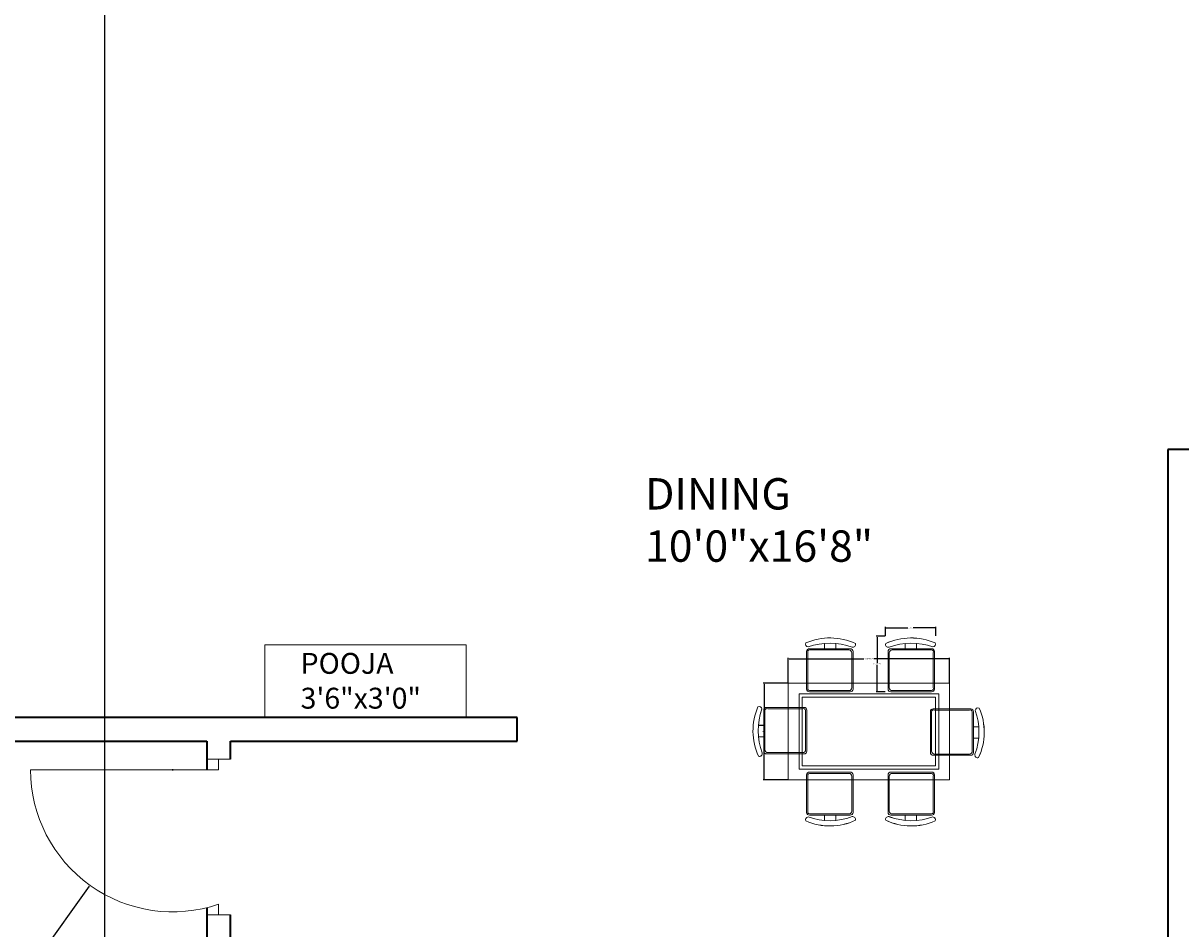
# Model space of a CAD drawing. Units: inches. Extents: x 1902 to 2626, y 1199 to 2408.
# Tile 3 of 9: x 2113 to 2334, y 1470 to 1644. Entities that reach past the tile are written whole.
import ezdxf

# ---------------------------------------------------------------- set-up
doc = ezdxf.new("R2010")
doc.units = ezdxf.units.IN
for name, color, linetype, lineweight in [('A-ANNO-DIMS', 2, 'Continuous', 18), ('A-AREA-IDEN', 7, 'Continuous', 18), ('A-DOOR', 31, 'Continuous', 18), ('A-FLOR-CASE', 8, 'Continuous', 18), ('A-FURN', 8, 'Continuous', 13), ('A-WALL', 7, 'Continuous', 35)]:
    doc.layers.add(name, color=color, linetype=linetype, lineweight=lineweight)
doc.styles.get("Standard").update_dxf_attribs({"font": 'arial.ttf'})
doc.dimstyles.get("Standard").update_dxf_attribs({"dimtxt": 0.18, "dimasz": 0.18, "dimexe": 0.18, "dimexo": 0.0625, "dimgap": 0.09, "dimtad": 0, "dimtih": 1, "dimtoh": 1, "dimdec": 4, "dimzin": 0, "dimdsep": 46, "dimtxsty": 'Standard', "dimcen": 0.09, "dimadec": 0, "dimazin": 0, "dimtfac": 1, "dimtdec": 4, "dimtofl": 0, "dimtmove": 0, "dimatfit": 3, "dimfxl": 1, "dimtolj": 1, "dimtzin": 0, "dimarcsym": 0})

# ---------------------------------------------------------------- blocks, each defined once
blk = doc.blocks.new('TABLE-DINING-RECT')
for points in [[(0, 18.51), (30.84, 18.51), (30.84, 0), (0, 0)], [(2.06, 16.45), (28.79, 16.45), (28.79, 2.06), (2.06, 2.06)], [(2.67, 15.83), (28.17, 15.83), (28.17, 2.67), (2.67, 2.67)]]:
    blk.add_lwpolyline(points, close=True)
blk = doc.blocks.new('CHAIR-DINING')
for points in [[(8.55, 2.06), (0.75, 2.06, -0.414214), (0.2, 2.6), (0.2, 9.77, -0.414214), (0.75, 10.32), (8.55, 10.32, -0.414214), (9.09, 9.77), (9.09, 2.6, -0.414214), (8.55, 2.06)], [(8.91, 1.78, -0.578392), (9.54, 1.08, -0.214524), (0.06, 0.96, -0.552014), (0.5, 1.72, 0.175809), (8.91, 1.78)], [(5.81, 2.06), (5.81, 1.07, 0.064759)]]:
    blk.add_lwpolyline(points, format="xyb")
blk.add_lwpolyline([(0.75, 2.3), (8.3, 2.3, 0.414214), (8.85, 2.85), (8.85, 9.53, 0.414214), (8.3, 10.07), (0.75, 10.07, 0.512069), (0.45, 9.53), (0.45, 2.85, 0.512069)], format="xyb", close=True)
blk.add_lwpolyline([(3.63, 1.05), (3.63, 2.06)])
blk = doc.blocks.new('*D12')
at = {"layer": 'A-ANNO-DIMS', "color": 0, "lineweight": -2, "transparency": 16777216}
for p, q in [((2259.21, 1517.35), (2259.21, 1522.1)), ((2259.39, 1521.92), (2273.67, 1521.92)), ((2289.87, 1521.92), (2275.6, 1521.92)), ((2290.05, 1517.35), (2290.05, 1522.1))]:
    blk.add_line(p, q, dxfattribs=at)
at = {"layer": 'A-ANNO-DIMS', "color": 0, "transparency": 16777216}
for points in [[(2259.39, 1521.95), (2259.39, 1521.89), (2259.21, 1521.92)], [(2289.87, 1521.95), (2289.87, 1521.89), (2290.05, 1521.92)]]:
    blk.add_solid(points, dxfattribs=at)
at = {"layer": 'Defpoints', "color": 0, "transparency": 16777216}
for p in [(2290.05, 1521.92), (2259.21, 1517.29), (2290.05, 1517.29)]:
    blk.add_point(p, dxfattribs=at)
at = {"layer": 'A-ANNO-DIMS', "color": 0, "transparency": 16777216, "insert": (2274.63, 1521.92), "char_height": 0.18, "attachment_point": 5}
blk.add_mtext('\\A1;TABLE 31 TYP.', dxfattribs=at)
blk = doc.blocks.new('*D13')
at = {"layer": 'A-ANNO-DIMS', "color": 0, "lineweight": -2, "transparency": 16777216}
for p, q in [((2259.15, 1517.29), (2254.4, 1517.29)), ((2254.58, 1517.11), (2254.58, 1508.22)), ((2254.58, 1498.96), (2254.58, 1507.85)), ((2259.15, 1498.78), (2254.4, 1498.78))]:
    blk.add_line(p, q, dxfattribs=at)
at = {"layer": 'A-ANNO-DIMS', "color": 0, "transparency": 16777216}
for points in [[(2254.55, 1517.11), (2254.61, 1517.11), (2254.58, 1517.29)], [(2254.55, 1498.96), (2254.61, 1498.96), (2254.58, 1498.78)]]:
    blk.add_solid(points, dxfattribs=at)
at = {"layer": 'Defpoints', "color": 0, "transparency": 16777216}
for p in [(2254.58, 1517.29), (2259.21, 1517.29), (2259.21, 1498.78)]:
    blk.add_point(p, dxfattribs=at)
at = {"layer": 'A-ANNO-DIMS', "color": 0, "transparency": 16777216, "insert": (2254.58, 1508.04), "char_height": 0.18, "attachment_point": 5}
blk.add_mtext('\\A1;19 TYP.', dxfattribs=at)
blk = doc.blocks.new('*D14')
at = {"layer": 'A-ANNO-DIMS', "color": 0, "lineweight": -2, "transparency": 16777216}
for p, q in [((2277.74, 1526.29), (2276.02, 1526.29)), ((2276.2, 1526.11), (2276.2, 1521.13)), ((2276.2, 1515.79), (2276.2, 1520.77)), ((2277.74, 1515.61), (2276.02, 1515.61))]:
    blk.add_line(p, q, dxfattribs=at)
at = {"layer": 'A-ANNO-DIMS', "color": 0, "transparency": 16777216}
for points in [[(2276.17, 1526.11), (2276.23, 1526.11), (2276.2, 1526.29)], [(2276.17, 1515.79), (2276.23, 1515.79), (2276.2, 1515.61)]]:
    blk.add_solid(points, dxfattribs=at)
at = {"layer": 'Defpoints', "color": 0, "transparency": 16777216}
for p in [(2277.8, 1526.29), (2276.2, 1515.61), (2277.8, 1515.61)]:
    blk.add_point(p, dxfattribs=at)
at = {"layer": 'A-ANNO-DIMS', "color": 0, "transparency": 16777216, "insert": (2276.2, 1520.95), "char_height": 0.18, "attachment_point": 5}
blk.add_mtext('\\A1;CHAIR 11 TYP.', dxfattribs=at)
blk = doc.blocks.new('*D15')
at = {"layer": 'A-ANNO-DIMS', "color": 0, "lineweight": -2, "transparency": 16777216}
for p, q in [((2277.8, 1526.35), (2277.8, 1528.07)), ((2277.98, 1527.89), (2282.1, 1527.89)), ((2287.25, 1527.89), (2283.14, 1527.89)), ((2287.43, 1526.35), (2287.43, 1528.07))]:
    blk.add_line(p, q, dxfattribs=at)
at = {"layer": 'A-ANNO-DIMS', "color": 0, "transparency": 16777216}
for points in [[(2277.98, 1527.92), (2277.98, 1527.86), (2277.8, 1527.89)], [(2287.25, 1527.92), (2287.25, 1527.86), (2287.43, 1527.89)]]:
    blk.add_solid(points, dxfattribs=at)
at = {"layer": 'Defpoints', "color": 0, "transparency": 16777216}
for p in [(2277.8, 1527.89), (2277.8, 1526.29), (2287.43, 1526.29)]:
    blk.add_point(p, dxfattribs=at)
at = {"layer": 'A-ANNO-DIMS', "color": 0, "transparency": 16777216, "insert": (2282.62, 1527.89), "char_height": 0.18, "attachment_point": 5}
blk.add_mtext('\\A1;10 TYP.', dxfattribs=at)
blk = doc.blocks.new('*D29')
at = {"layer": 'A-ANNO-DIMS', "color": 0, "lineweight": -2, "transparency": 16777216}
for p, q in [((2191.29, 2322.47), (1943.87, 2322.47)), ((1944.05, 2322.29), (1944.05, 1836.38)), ((1944.05, 1350.11), (1944.05, 1836.02)), ((2202.79, 1349.93), (1943.87, 1349.93))]:
    blk.add_line(p, q, dxfattribs=at)
at = {"layer": 'A-ANNO-DIMS', "color": 0, "transparency": 16777216}
for points in [[(1944.02, 2322.29), (1944.08, 2322.29), (1944.05, 2322.47)], [(1944.02, 1350.11), (1944.08, 1350.11), (1944.05, 1349.93)]]:
    blk.add_solid(points, dxfattribs=at)
at = {"layer": 'Defpoints', "color": 0, "transparency": 16777216}
for p in [(1944.05, 2322.47), (2191.35, 2322.47), (2202.85, 1349.93)]:
    blk.add_point(p, dxfattribs=at)
at = {"layer": 'A-ANNO-DIMS', "color": 0, "transparency": 16777216, "insert": (1944.05, 1836.2), "char_height": 0.18, "attachment_point": 5}
blk.add_mtext('\\A1;972.5', dxfattribs=at)
blk = doc.blocks.new('*D38')
at = {"layer": 'A-ANNO-DIMS', "color": 0, "lineweight": -2, "transparency": 16777216}
for p, q in [((2008.35, 1874.05), (2008.35, 1198.67)), ((2128.35, 1874.05), (2128.35, 1198.67)), ((2008.53, 1198.85), (2068.07, 1198.85)), ((2128.17, 1198.85), (2068.63, 1198.85))]:
    blk.add_line(p, q, dxfattribs=at)
at = {"layer": 'A-ANNO-DIMS', "color": 0, "transparency": 16777216}
for points in [[(2008.53, 1198.88), (2008.53, 1198.82), (2008.35, 1198.85)], [(2128.17, 1198.88), (2128.17, 1198.82), (2128.35, 1198.85)]]:
    blk.add_solid(points, dxfattribs=at)
at = {"layer": 'Defpoints', "color": 0, "transparency": 16777216}
for p in [(2008.35, 1874.11), (2128.35, 1874.11), (2128.35, 1198.85)]:
    blk.add_point(p, dxfattribs=at)
at = {"layer": 'A-ANNO-DIMS', "color": 0, "transparency": 16777216, "insert": (2068.35, 1198.85), "char_height": 0.18, "attachment_point": 5}
blk.add_mtext('\\A1;120', dxfattribs=at)
blk = doc.blocks.new('*D51')
at = {"layer": 'A-ANNO-DIMS', "color": 0, "lineweight": -2, "transparency": 16777216}
for p, q in [((2141.3, 1500.7), (2141.48, 1500.7)), ((2141.39, 1500.61), (2141.39, 1500.79)), ((2116.07, 1465.29), (2125.46, 1478.42)), ((2115.89, 1465.29), (2116.07, 1465.29))]:
    blk.add_line(p, q, dxfattribs=at)
at = {"layer": 'A-ANNO-DIMS', "color": 0, "transparency": 16777216}
blk.add_solid([(2125.44, 1478.44), (2125.49, 1478.4), (2125.57, 1478.57)], dxfattribs=at)
at = {"layer": 'Defpoints', "color": 0, "transparency": 16777216}
for p in [(2141.39, 1500.7), (2125.57, 1478.57)]:
    blk.add_point(p, dxfattribs=at)
at = {"layer": 'A-ANNO-DIMS', "color": 0, "transparency": 16777216, "insert": (2115.34, 1465.29), "char_height": 0.18, "attachment_point": 5}
blk.add_mtext('\\A1;R27.204', dxfattribs=at)

msp = doc.modelspace()

# ---------------------------------------------------------------- linework, layer by layer
at = {"layer": 'A-DOOR'}
for p, q in [((2152.4363, 1502.6974), (2147.9363, 1502.6974)), ((2147.9363, 1502.6974), (2150.1863, 1502.6974)), ((2150.1863, 1502.6974), (2150.1863, 1502.6974)), ((2150.1863, 1502.6974), (2150.1863, 1500.6974)), ((2150.1863, 1500.6974), (2114.1863, 1500.6974)), ((2150.1863, 1472.9548), (2150.1863, 1474.9548)), ((2147.9363, 1472.9548), (2152.4363, 1472.9548)), ((2152.4363, 1472.9548), (2150.1863, 1472.9548))]:
    msp.add_line(p, q, dxfattribs=at)
msp.add_arc((2141.3902, 1500.6974), 27.2039, 180, 288.865006, dxfattribs=at)
at = {"layer": 'A-FLOR-CASE'}
msp.add_lwpolyline([(2159.0496, 1524.6144), (2197.5917, 1524.6144), (2197.5917, 1510.7028), (2159.0496, 1510.7028)], close=True, dxfattribs=at)
at = {"layer": 'A-FURN'}
for points in [[(2263.0262, 1524.2123, -0.17580919), (2271.427, 1524.1486, 0.57839206), (2272.0634, 1524.8484, 0.21452438), (2262.5807, 1524.9757, 0.55201397), (2263.0262, 1524.2123, -0.06507904)], [(2263.0262, 1524.2123, -0.17580919), (2271.427, 1524.1486, 0.57839206), (2272.0634, 1524.8484, 0.21452438), (2262.5807, 1524.9757, 0.55201397), (2263.0262, 1524.2123, -0.06507904)], [(2263.0262, 1524.2119, -0.17580919), (2271.427, 1524.1483, 0.57839206), (2272.0635, 1524.8481, 0.21452438), (2262.5807, 1524.9754, 0.55201397), (2263.0262, 1524.2119, -0.06507904)], [(2263.0262, 1524.2119, -0.17580919), (2271.427, 1524.1483, 0.57839206), (2272.0635, 1524.8481, 0.21452438), (2262.5807, 1524.9754, 0.55201397), (2263.0262, 1524.2119, -0.06507904)], [(2268.3312, 1523.8751), (2268.3312, 1524.8614, -0.06475861)], [(2268.3312, 1523.8751), (2268.3312, 1524.8614, -0.06475861)], [(2268.3312, 1523.8748), (2268.3312, 1524.8611, -0.06475861)], [(2268.3312, 1523.8748), (2268.3312, 1524.8611, -0.06475861)], [(2278.4995, 1524.1486, -0.57839206), (2277.863, 1524.8484, -0.21452438), (2287.3458, 1524.9757, -0.55201397), (2286.9003, 1524.2123, 0.1758092), (2278.4995, 1524.1486)], [(2278.4995, 1524.1486, -0.57839206), (2277.863, 1524.8484, -0.21452438), (2287.3458, 1524.9757, -0.55201397), (2286.9003, 1524.2123, 0.1758092), (2278.4995, 1524.1486)], [(2278.4995, 1524.1483, -0.57839206), (2277.863, 1524.8481, -0.21452438), (2287.3458, 1524.9754, -0.55201397), (2286.9003, 1524.2119, 0.1758092), (2278.4995, 1524.1483)], [(2281.5953, 1523.8751), (2281.5953, 1524.8614, 0.06475861)], [(2281.5953, 1523.8751), (2281.5953, 1524.8614, 0.06475861)], [(2281.5953, 1523.8748), (2281.5953, 1524.8611, 0.06475861)], [(2271.0706, 1523.8751), (2263.2715, 1523.8751, 0.41421356), (2262.7259, 1523.3295), (2262.7259, 1516.1584, 0.41421356), (2263.2715, 1515.6127), (2271.0706, 1515.6127, 0.41421356), (2271.6162, 1516.1584), (2271.6162, 1523.3295, 0.41421356), (2271.0706, 1523.8751)], [(2271.0706, 1523.8751), (2263.2715, 1523.8751, 0.41421356), (2262.7259, 1523.3295), (2262.7259, 1516.1584, 0.41421356), (2263.2715, 1515.6127), (2271.0706, 1515.6127, 0.41421356), (2271.6162, 1516.1584), (2271.6162, 1523.3295, 0.41421356), (2271.0706, 1523.8751)], [(2271.0706, 1523.8748), (2263.2716, 1523.8748, 0.41421356), (2262.7259, 1523.3291), (2262.7259, 1516.158, 0.41421356), (2263.2716, 1515.6124), (2271.0706, 1515.6124, 0.41421356), (2271.6163, 1516.158), (2271.6163, 1523.3291, 0.41421356), (2271.0706, 1523.8748)], [(2271.0706, 1523.8748), (2263.2716, 1523.8748, 0.41421356), (2262.7259, 1523.3291), (2262.7259, 1516.158, 0.41421356), (2263.2716, 1515.6124), (2271.0706, 1515.6124, 0.41421356), (2271.6163, 1516.158), (2271.6163, 1523.3291, 0.41421356), (2271.0706, 1523.8748)], [(2286.6549, 1523.8751, -0.41421356), (2287.2006, 1523.3295), (2287.2006, 1516.1584, -0.41421356), (2286.6549, 1515.6127), (2278.8559, 1515.6127, -0.41421356), (2278.3102, 1516.1584), (2278.3102, 1523.3295, -0.41421356), (2278.8559, 1523.8751), (2286.6549, 1523.8751)], [(2286.6549, 1523.8751, -0.41421356), (2287.2006, 1523.3295), (2287.2006, 1516.1584, -0.41421356), (2286.6549, 1515.6127), (2278.8559, 1515.6127, -0.41421356), (2278.3102, 1516.1584), (2278.3102, 1523.3295, -0.41421356), (2278.8559, 1523.8751), (2286.6549, 1523.8751)], [(2286.6549, 1523.8748, -0.41421356), (2287.2006, 1523.3291), (2287.2006, 1516.158, -0.41421356), (2286.6549, 1515.6124), (2278.8559, 1515.6124, -0.41421356), (2278.3102, 1516.158), (2278.3102, 1523.3291, -0.41421356), (2278.8559, 1523.8748), (2286.6549, 1523.8748)], [(2254.2373, 1503.9255, -0.57839206), (2253.5375, 1503.289, -0.21452438), (2253.4102, 1512.7718, -0.55201397), (2254.1736, 1512.3263, 0.17580937), (2254.2373, 1503.9255)], [(2254.2373, 1503.9255, -0.57839206), (2253.5375, 1503.289, -0.21452438), (2253.4102, 1512.7718, -0.55201397), (2254.1736, 1512.3263, 0.17580937), (2254.2373, 1503.9255)], [(2254.5108, 1512.0809, -0.41421356), (2255.0564, 1512.6266), (2262.2275, 1512.6266, -0.41421356), (2262.7732, 1512.0809), (2262.7732, 1504.2819, -0.41421356), (2262.2275, 1503.7363), (2255.0564, 1503.7363, -0.41421356), (2254.5108, 1504.2819), (2254.5108, 1512.0809)], [(2254.5108, 1512.0809, -0.41421356), (2255.0564, 1512.6266), (2262.2275, 1512.6266, -0.41421356), (2262.7732, 1512.0809), (2262.7732, 1504.2819, -0.41421356), (2262.2275, 1503.7363), (2255.0564, 1503.7363, -0.41421356), (2254.5108, 1504.2819), (2254.5108, 1512.0809)], [(2294.6724, 1511.8135, 0.41421356), (2294.1267, 1512.3592), (2286.9557, 1512.3592, 0.41421356), (2286.41, 1511.8135), (2286.41, 1504.0145, 0.41421356), (2286.9557, 1503.4688), (2294.1267, 1503.4688, 0.41421356), (2294.6724, 1504.0145), (2294.6724, 1511.8135)], [(2295.0095, 1512.0589, -0.17580919), (2294.9459, 1503.658, 0.57839206), (2295.6457, 1503.0216, 0.21452438), (2295.773, 1512.5044, 0.55201397), (2295.0095, 1512.0589, -0.06507904)], [(2254.5108, 1507.0213), (2253.5245, 1507.0213, 0.06475861)], [(2254.5108, 1507.0213), (2253.5245, 1507.0213, 0.06475861)], [(2294.6724, 1506.7539), (2295.6587, 1506.7539, -0.06475861)], [(2271.0706, 1491.9978), (2263.2715, 1491.9978, -0.41421356), (2262.7259, 1492.5435), (2262.7259, 1499.7145, -0.41421356), (2263.2715, 1500.2602), (2271.0706, 1500.2602, -0.41421356), (2271.6162, 1499.7145), (2271.6162, 1492.5435, -0.41421356), (2271.0706, 1491.9978)], [(2271.0706, 1491.9978), (2263.2715, 1491.9978, -0.41421356), (2262.7259, 1492.5435), (2262.7259, 1499.7145, -0.41421356), (2263.2715, 1500.2602), (2271.0706, 1500.2602, -0.41421356), (2271.6162, 1499.7145), (2271.6162, 1492.5435, -0.41421356), (2271.0706, 1491.9978)], [(2271.0706, 1491.9975), (2263.2716, 1491.9975, -0.41421356), (2262.7259, 1492.5431), (2262.7259, 1499.7142, -0.41421356), (2263.2716, 1500.2599), (2271.0706, 1500.2599, -0.41421356), (2271.6163, 1499.7142), (2271.6163, 1492.5431, -0.41421356), (2271.0706, 1491.9975)], [(2271.0706, 1491.9975), (2263.2716, 1491.9975, -0.41421356), (2262.7259, 1492.5431), (2262.7259, 1499.7142, -0.41421356), (2263.2716, 1500.2599), (2271.0706, 1500.2599, -0.41421356), (2271.6163, 1499.7142), (2271.6163, 1492.5431, -0.41421356), (2271.0706, 1491.9975)], [(2286.6549, 1491.9978, 0.41421356), (2287.2006, 1492.5435), (2287.2006, 1499.7145, 0.41421356), (2286.6549, 1500.2602), (2278.8559, 1500.2602, 0.41421356), (2278.3102, 1499.7145), (2278.3102, 1492.5435, 0.41421356), (2278.8559, 1491.9978), (2286.6549, 1491.9978)], [(2286.6549, 1491.9975, 0.41421356), (2287.2006, 1492.5431), (2287.2006, 1499.7142, 0.41421356), (2286.6549, 1500.2599), (2278.8559, 1500.2599, 0.41421356), (2278.3102, 1499.7142), (2278.3102, 1492.5431, 0.41421356), (2278.8559, 1491.9975), (2286.6549, 1491.9975)], [(2271.427, 1491.7243, -0.57839206), (2272.0634, 1491.0245, -0.21452438), (2262.5807, 1490.8972, -0.55201397), (2263.0262, 1491.6607, 0.17580929), (2271.427, 1491.7243)], [(2271.427, 1491.7243, -0.57839206), (2272.0634, 1491.0245, -0.21452438), (2262.5807, 1490.8972, -0.55201397), (2263.0262, 1491.6607, 0.17580929), (2271.427, 1491.7243)], [(2271.427, 1491.7239, -0.57839206), (2272.0635, 1491.0241, -0.21452438), (2262.5807, 1490.8969, -0.55201397), (2263.0262, 1491.6603, 0.17580929), (2271.427, 1491.7239)], [(2271.427, 1491.7239, -0.57839206), (2272.0635, 1491.0241, -0.21452438), (2262.5807, 1490.8969, -0.55201397), (2263.0262, 1491.6603, 0.17580929), (2271.427, 1491.7239)], [(2268.3312, 1491.9978), (2268.3312, 1491.0115, 0.06475861)], [(2268.3312, 1491.9978), (2268.3312, 1491.0115, 0.06475861)], [(2268.3312, 1491.9975), (2268.3312, 1491.0112, 0.06475861)], [(2268.3312, 1491.9975), (2268.3312, 1491.0112, 0.06475861)], [(2286.9003, 1491.6607, -0.17580928), (2278.4995, 1491.7243, 0.57839206), (2277.863, 1491.0245, 0.21452438), (2287.3458, 1490.8972, 0.55201397), (2286.9003, 1491.6607, -0.06507904)], [(2286.9003, 1491.6603, -0.17580928), (2278.4995, 1491.7239, 0.57839206), (2277.863, 1491.0241, 0.21452438), (2287.3458, 1490.8969, 0.55201397), (2286.9003, 1491.6603, -0.06507904)], [(2281.5953, 1491.9978), (2281.5953, 1491.0115, -0.06475861)], [(2281.5953, 1491.9975), (2281.5953, 1491.0112, -0.06475861)]]:
    msp.add_lwpolyline(points, format="xyb", dxfattribs=at)
for points in [[(2266.1481, 1524.8793), (2266.1481, 1523.8751)], [(2266.1481, 1524.8793), (2266.1481, 1523.8751)], [(2266.1481, 1524.879), (2266.1481, 1523.8748)], [(2266.1481, 1524.879), (2266.1481, 1523.8748)], [(2283.7784, 1524.8793), (2283.7784, 1523.8751)], [(2283.7784, 1524.8793), (2283.7784, 1523.8751)], [(2283.7784, 1524.879), (2283.7784, 1523.8748)], [(2253.5065, 1509.2044), (2254.5108, 1509.2044)], [(2253.5065, 1509.2044), (2254.5108, 1509.2044)], [(2295.6766, 1508.937), (2294.6724, 1508.937)], [(2266.1481, 1490.9936), (2266.1481, 1491.9978)], [(2266.1481, 1490.9936), (2266.1481, 1491.9978)], [(2266.1481, 1490.9932), (2266.1481, 1491.9975)], [(2266.1481, 1490.9932), (2266.1481, 1491.9975)], [(2283.7784, 1490.9936), (2283.7784, 1491.9978)], [(2283.7784, 1490.9932), (2283.7784, 1491.9975)]]:
    msp.add_lwpolyline(points, dxfattribs=at)
for points in [[(2263.2748, 1523.6293), (2270.8248, 1523.6293, -0.41421356), (2271.3704, 1523.0836), (2271.3704, 1516.4042, -0.41421356), (2270.8248, 1515.8585), (2263.2748, 1515.8585, -0.51206948), (2262.9717, 1516.4042), (2262.9717, 1523.0836, -0.51206948)], [(2263.2748, 1523.6293), (2270.8248, 1523.6293, -0.41421356), (2271.3704, 1523.0836), (2271.3704, 1516.4042, -0.41421356), (2270.8248, 1515.8585), (2263.2748, 1515.8585, -0.51206948), (2262.9717, 1516.4042), (2262.9717, 1523.0836, -0.51206948)], [(2263.2749, 1523.6289), (2270.8248, 1523.6289, -0.41421356), (2271.3704, 1523.0833), (2271.3704, 1516.4038, -0.41421356), (2270.8248, 1515.8582), (2263.2749, 1515.8582, -0.51206948), (2262.9717, 1516.4038), (2262.9717, 1523.0833, -0.51206948)], [(2263.2749, 1523.6289), (2270.8248, 1523.6289, -0.41421356), (2271.3704, 1523.0833), (2271.3704, 1516.4038, -0.41421356), (2270.8248, 1515.8582), (2263.2749, 1515.8582, -0.51206948), (2262.9717, 1516.4038), (2262.9717, 1523.0833, -0.51206948)], [(2286.6516, 1523.6293), (2279.1017, 1523.6293, 0.41421356), (2278.556, 1523.0836), (2278.556, 1516.4042, 0.41421356), (2279.1017, 1515.8585), (2286.6516, 1515.8585, 0.51206948), (2286.9547, 1516.4042), (2286.9547, 1523.0836, 0.51206948)], [(2286.6516, 1523.6293), (2279.1017, 1523.6293, 0.41421356), (2278.556, 1523.0836), (2278.556, 1516.4042, 0.41421356), (2279.1017, 1515.8585), (2286.6516, 1515.8585, 0.51206948), (2286.9547, 1516.4042), (2286.9547, 1523.0836, 0.51206948)], [(2286.6516, 1523.6289), (2279.1017, 1523.6289, 0.41421356), (2278.5561, 1523.0833), (2278.5561, 1516.4038, 0.41421356), (2279.1017, 1515.8582), (2286.6516, 1515.8582, 0.51206948), (2286.9548, 1516.4038), (2286.9548, 1523.0833, 0.51206948)], [(2254.7566, 1512.0776), (2254.7566, 1504.5277, 0.41421356), (2255.3023, 1503.9821), (2261.9817, 1503.9821, 0.41421356), (2262.5274, 1504.5277), (2262.5274, 1512.0776, 0.51206948), (2261.9817, 1512.3808), (2255.3023, 1512.3808, 0.51206948)], [(2254.7566, 1512.0776), (2254.7566, 1504.5277, 0.41421356), (2255.3023, 1503.9821), (2261.9817, 1503.9821, 0.41421356), (2262.5274, 1504.5277), (2262.5274, 1512.0776, 0.51206948), (2261.9817, 1512.3808), (2255.3023, 1512.3808, 0.51206948)], [(2294.4266, 1511.8102), (2294.4266, 1504.2603, -0.41421356), (2293.8809, 1503.7146), (2287.2015, 1503.7146, -0.41421356), (2286.6558, 1504.2603), (2286.6558, 1511.8102, -0.51206948), (2287.2015, 1512.1133), (2293.8809, 1512.1133, -0.51206948)], [(2263.2748, 1492.2436), (2270.8248, 1492.2436, 0.41421356), (2271.3704, 1492.7893), (2271.3704, 1499.4687, 0.41421356), (2270.8248, 1500.0144), (2263.2748, 1500.0144, 0.51206948), (2262.9717, 1499.4687), (2262.9717, 1492.7893, 0.51206948)], [(2263.2748, 1492.2436), (2270.8248, 1492.2436, 0.41421356), (2271.3704, 1492.7893), (2271.3704, 1499.4687, 0.41421356), (2270.8248, 1500.0144), (2263.2748, 1500.0144, 0.51206948), (2262.9717, 1499.4687), (2262.9717, 1492.7893, 0.51206948)], [(2263.2749, 1492.2433), (2270.8248, 1492.2433, 0.41421356), (2271.3704, 1492.7889), (2271.3704, 1499.4684, 0.41421356), (2270.8248, 1500.014), (2263.2749, 1500.014, 0.51206948), (2262.9717, 1499.4684), (2262.9717, 1492.7889, 0.51206948)], [(2263.2749, 1492.2433), (2270.8248, 1492.2433, 0.41421356), (2271.3704, 1492.7889), (2271.3704, 1499.4684, 0.41421356), (2270.8248, 1500.014), (2263.2749, 1500.014, 0.51206948), (2262.9717, 1499.4684), (2262.9717, 1492.7889, 0.51206948)], [(2286.6516, 1492.2436), (2279.1017, 1492.2436, -0.41421356), (2278.556, 1492.7893), (2278.556, 1499.4687, -0.41421356), (2279.1017, 1500.0144), (2286.6516, 1500.0144, -0.51206948), (2286.9547, 1499.4687), (2286.9547, 1492.7893, -0.51206948)], [(2286.6516, 1492.2433), (2279.1017, 1492.2433, -0.41421356), (2278.5561, 1492.7889), (2278.5561, 1499.4684, -0.41421356), (2279.1017, 1500.014), (2286.6516, 1500.014, -0.51206948), (2286.9548, 1499.4684), (2286.9548, 1492.7889, -0.51206948)]]:
    msp.add_lwpolyline(points, format="xyb", close=True, dxfattribs=at)
at = {"layer": 'A-WALL'}
for p, q in [((2331.8507, 1561.9733), (2331.8507, 1404.4733)), ((2340.3371, 1561.9733), (2331.8507, 1561.9733)), ((2207.3507, 1510.7028), (2008.3507, 1510.7028)), ((2207.3507, 1506.2028), (2207.3507, 1510.7028)), ((2008.3507, 1506.2028), (2118.3507, 1506.2028)), ((2118.3507, 1506.2028), (2147.9363, 1506.2028)), ((2147.9363, 1506.2028), (2147.9363, 1500.6974)), ((2152.4363, 1506.2028), (2207.3507, 1506.2028)), ((2152.4363, 1502.6974), (2152.4363, 1506.2028)), ((2147.9363, 1474.2928), (2147.9363, 1467.7028)), ((2152.4363, 1467.7028), (2152.4363, 1472.9548))]:
    msp.add_line(p, q, dxfattribs=at)

# ---------------------------------------------------------------- block references
at = {"layer": 'A-FURN'}
for p, rotation in [((2287.4052, 1525.9314), 180), ((2252.4542, 1512.8309), 270), ((2252.4542, 1512.8309), 270)]:
    msp.add_blockref('CHAIR-DINING', p, dxfattribs=dict(at, rotation=rotation))
for p in [(2259.2113, 1498.7809), (2259.2113, 1498.7809), (2259.2113, 1498.7806), (2259.2113, 1498.7806)]:
    msp.add_blockref('TABLE-DINING-RECT', p, dxfattribs=at)
at = {"layer": 'A-FURN', "extrusion": (0, 0, -1), "zscale": -1, "rotation": 270}
for p in [(-2296.729, 1512.5641), (-2296.729, 1512.5641), (-2296.729, 1512.5638)]:
    msp.add_blockref('CHAIR-DINING', p, dxfattribs=at)
at = {"layer": 'A-FURN', "extrusion": (0, 0, -1), "zscale": -1}
for p in [(-2287.4052, 1489.9412), (-2287.4052, 1489.9409)]:
    msp.add_blockref('CHAIR-DINING', p, dxfattribs=at)

# ---------------------------------------------------------------- texts
at = {"layer": 'A-AREA-IDEN', "attachment_point": 1}
for s, width, insert, char_height in [('DINING\\P10\'0"x16\'8"', 110.849605, (2231.804, 1556.517), 6), ('POOJA\\P3\'6"x3\'0"', 80.559014, (2165.8731, 1523.0648), 4)]:
    msp.add_mtext_dynamic_manual_height_columns(s, width=width, gutter_width=12.5, heights=[0], dxfattribs=dict(at, insert=insert, char_height=char_height))

# ---------------------------------------------------------------- dimensions: what is measured, and where the dimension line sits
at = {"layer": 'A-ANNO-DIMS'}
dim = msp.add_linear_dim(base=(1944.0507, 2322.4733), p1=(2202.8507, 1349.9322), p2=(2191.3507, 2322.4733), angle=90, dimstyle='Standard', override={"dimdec": 1, "dimlfac": 1, "dimrnd": 0, "dimzin": 0, "dimdsep": 46, "dimlunit": 2}, dxfattribs=at)
dim.commit()
dim.dimension.update_dxf_attribs({"geometry": '*D29', "text_midpoint": (1944.0507, 1836.2028)})
dim = msp.add_linear_dim(base=(2128.3507, 1198.8475), p1=(2008.3507, 1874.11), p2=(2128.3507, 1874.11), dimstyle='Standard', override={"dimdec": 0, "dimlfac": 1, "dimrnd": 0, "dimzin": 0, "dimdsep": 46, "dimlunit": 2}, dxfattribs=at)
dim.commit()
dim.dimension.update_dxf_attribs({"geometry": '*D38', "text_midpoint": (2068.3507, 1198.8475)})
for base, p1, p2, angle, text, picture, middle in [((2277.8033, 1527.8929), (2287.4288, 1526.2911), (2277.8033, 1526.2911), 180, '<> TYP.', '*D15', (2282.6161, 1527.8929)), ((2276.2015, 1515.6124), (2277.8033, 1526.2911), (2277.8033, 1515.6124), 270, 'CHAIR <> TYP.', '*D14', (2276.2015, 1520.9517)), ((2254.5847, 1517.2886), (2259.2112, 1498.7826), (2259.2112, 1517.2886), 90, '<> TYP.', '*D13', (2254.5847, 1508.0356))]:
    dim = msp.add_linear_dim(base=base, p1=p1, p2=p2, angle=angle, text=text, dimstyle='Standard', override={"dimdec": 0, "dimlfac": 1, "dimrnd": 0, "dimzin": 0, "dimdsep": 46, "dimlunit": 2}, dxfattribs=at)
    dim.commit()
    dim.dimension.update_dxf_attribs({"geometry": picture, "text_midpoint": middle})
dim = msp.add_linear_dim(base=(2290.0545, 1521.9151), p1=(2259.2112, 1517.2886), p2=(2290.0545, 1517.2886), text='TABLE <> TYP.', dimstyle='Standard', override={"dimdec": 0, "dimlfac": 1, "dimrnd": 0, "dimzin": 0, "dimdsep": 46, "dimlunit": 2}, dxfattribs=at)
dim.commit()
dim.dimension.update_dxf_attribs({"geometry": '*D12', "text_midpoint": (2274.6328, 1521.9151)})
dim = msp.add_radius_dim(center=(2141.3902, 1500.6974), mpoint=(2125.5668, 1478.5688), dimstyle='Standard', override={"dimdec": 3, "dimlfac": 1, "dimrnd": 0, "dimzin": 0, "dimdsep": 46, "dimlunit": 2}, dxfattribs=at)
dim.commit()
dim.dimension.update_dxf_attribs({"geometry": '*D51', "text_midpoint": (2115.3434, 1465.2916), "dimtype": 164})

doc.saveas('drawing.dxf')
